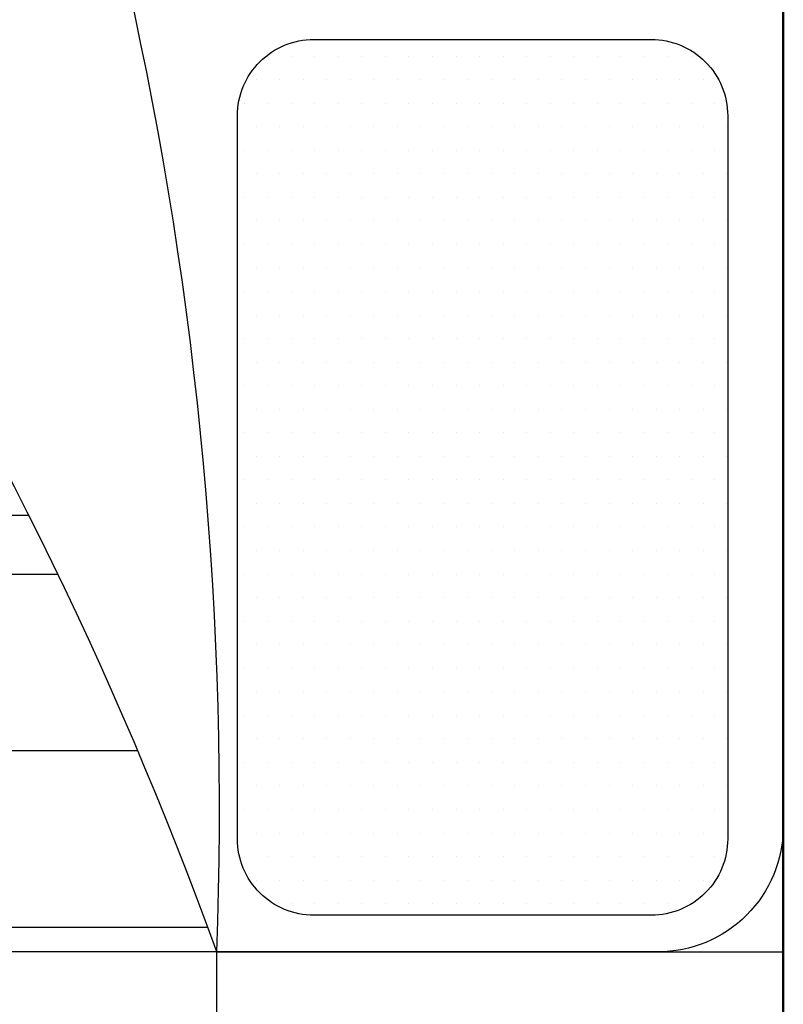
# Model space of a CAD drawing. Units: inches. Extents: x 3064 to 19385, y 846 to 15425.
# Tile 69 of 108: x 6580 to 6604, y 1624 to 1655. Entities that reach past the tile are written whole.
import ezdxf

# ---------------------------------------------------------------- set-up
doc = ezdxf.new("R2010")
doc.units = ezdxf.units.IN
doc.layers.add('A-FLOR-FIXT', color=9, linetype='Continuous', lineweight=18)
doc.layers.add('A-WALL', color=7, linetype='Continuous', lineweight=50)
doc.layers.add('BLOCK', color=6, linetype='Continuous')

# ---------------------------------------------------------------- blocks, each defined once
blk = doc.blocks.new('*X6')
at = {"color": 0}
for p, q in [((280.3125, 439.8862), (280.3125, 452.8965)), ((278.9062, 439.4824), (278.9062, 452.3385)), ((277.5, 439.4824), (277.5, 451.7019)), ((277.0312, 439.4824), (277.0312, 451.4714))]:
    blk.add_line(p, q, dxfattribs=at)
blk = doc.blocks.new('*X7')
at = {"color": 0}
for p, q in [((273.9375, 457.03125), (273.9375, 457.03125)), ((274.3125, 457.03125), (274.3125, 457.03125)), ((274.6875, 457.03125), (274.6875, 457.03125)), ((275.0625, 457.03125), (275.0625, 457.03125)), ((275.4375, 457.03125), (275.4375, 457.03125)), ((275.8125, 457.03125), (275.8125, 457.03125)), ((276.1875, 457.03125), (276.1875, 457.03125)), ((276.5625, 457.03125), (276.5625, 457.03125)), ((276.9375, 457.03125), (276.9375, 457.03125)), ((277.3125, 457.03125), (277.3125, 457.03125)), ((277.6875, 457.03125), (277.6875, 457.03125)), ((278.0625, 457.03125), (278.0625, 457.03125)), ((278.4375, 457.03125), (278.4375, 457.03125)), ((278.8125, 457.03125), (278.8125, 457.03125)), ((279.1875, 457.03125), (279.1875, 457.03125)), ((279.5625, 457.03125), (279.5625, 457.03125)), ((273.75, 456.9375), (273.75, 456.9375)), ((274.125, 456.9375), (274.125, 456.9375)), ((274.5, 456.9375), (274.5, 456.9375)), ((274.875, 456.9375), (274.875, 456.9375)), ((275.25, 456.9375), (275.25, 456.9375)), ((275.625, 456.9375), (275.625, 456.9375)), ((276, 456.9375), (276, 456.9375)), ((276.375, 456.9375), (276.375, 456.9375)), ((276.75, 456.9375), (276.75, 456.9375)), ((277.125, 456.9375), (277.125, 456.9375)), ((277.5, 456.9375), (277.5, 456.9375)), ((277.875, 456.9375), (277.875, 456.9375)), ((278.25, 456.9375), (278.25, 456.9375)), ((278.625, 456.9375), (278.625, 456.9375)), ((279, 456.9375), (279, 456.9375)), ((279.375, 456.9375), (279.375, 456.9375)), ((279.75, 456.9375), (279.75, 456.9375)), ((273.5625, 456.84375), (273.5625, 456.84375)), ((273.9375, 456.84375), (273.9375, 456.84375)), ((274.3125, 456.84375), (274.3125, 456.84375)), ((274.6875, 456.84375), (274.6875, 456.84375)), ((275.0625, 456.84375), (275.0625, 456.84375)), ((275.4375, 456.84375), (275.4375, 456.84375)), ((275.8125, 456.84375), (275.8125, 456.84375)), ((276.1875, 456.84375), (276.1875, 456.84375)), ((276.5625, 456.84375), (276.5625, 456.84375)), ((276.9375, 456.84375), (276.9375, 456.84375)), ((277.3125, 456.84375), (277.3125, 456.84375)), ((277.6875, 456.84375), (277.6875, 456.84375)), ((278.0625, 456.84375), (278.0625, 456.84375)), ((278.4375, 456.84375), (278.4375, 456.84375)), ((278.8125, 456.84375), (278.8125, 456.84375)), ((279.1875, 456.84375), (279.1875, 456.84375)), ((279.5625, 456.84375), (279.5625, 456.84375)), ((279.9375, 456.84375), (279.9375, 456.84375)), ((273.375, 456.75), (273.375, 456.75)), ((273.75, 456.75), (273.75, 456.75)), ((274.125, 456.75), (274.125, 456.75)), ((274.5, 456.75), (274.5, 456.75)), ((274.875, 456.75), (274.875, 456.75)), ((275.25, 456.75), (275.25, 456.75)), ((275.625, 456.75), (275.625, 456.75)), ((276, 456.75), (276, 456.75)), ((276.375, 456.75), (276.375, 456.75)), ((276.75, 456.75), (276.75, 456.75)), ((277.125, 456.75), (277.125, 456.75)), ((277.5, 456.75), (277.5, 456.75)), ((277.875, 456.75), (277.875, 456.75)), ((278.25, 456.75), (278.25, 456.75)), ((278.625, 456.75), (278.625, 456.75)), ((279, 456.75), (279, 456.75)), ((279.375, 456.75), (279.375, 456.75)), ((279.75, 456.75), (279.75, 456.75)), ((280.125, 456.75), (280.125, 456.75)), ((273.5625, 456.65625), (273.5625, 456.65625)), ((273.9375, 456.65625), (273.9375, 456.65625)), ((274.3125, 456.65625), (274.3125, 456.65625)), ((274.6875, 456.65625), (274.6875, 456.65625)), ((275.0625, 456.65625), (275.0625, 456.65625)), ((275.4375, 456.65625), (275.4375, 456.65625)), ((275.8125, 456.65625), (275.8125, 456.65625)), ((276.1875, 456.65625), (276.1875, 456.65625)), ((276.5625, 456.65625), (276.5625, 456.65625)), ((276.9375, 456.65625), (276.9375, 456.65625)), ((277.3125, 456.65625), (277.3125, 456.65625)), ((277.6875, 456.65625), (277.6875, 456.65625)), ((278.0625, 456.65625), (278.0625, 456.65625)), ((278.4375, 456.65625), (278.4375, 456.65625)), ((278.8125, 456.65625), (278.8125, 456.65625)), ((279.1875, 456.65625), (279.1875, 456.65625)), ((279.5625, 456.65625), (279.5625, 456.65625)), ((279.9375, 456.65625), (279.9375, 456.65625)), ((273.375, 456.5625), (273.375, 456.5625)), ((273.75, 456.5625), (273.75, 456.5625)), ((274.125, 456.5625), (274.125, 456.5625)), ((274.5, 456.5625), (274.5, 456.5625)), ((274.875, 456.5625), (274.875, 456.5625)), ((275.25, 456.5625), (275.25, 456.5625)), ((275.625, 456.5625), (275.625, 456.5625)), ((276, 456.5625), (276, 456.5625)), ((276.375, 456.5625), (276.375, 456.5625)), ((276.75, 456.5625), (276.75, 456.5625)), ((277.125, 456.5625), (277.125, 456.5625)), ((277.5, 456.5625), (277.5, 456.5625)), ((277.875, 456.5625), (277.875, 456.5625)), ((278.25, 456.5625), (278.25, 456.5625)), ((278.625, 456.5625), (278.625, 456.5625)), ((279, 456.5625), (279, 456.5625)), ((279.375, 456.5625), (279.375, 456.5625)), ((279.75, 456.5625), (279.75, 456.5625)), ((280.125, 456.5625), (280.125, 456.5625)), ((273.5625, 456.46875), (273.5625, 456.46875)), ((273.9375, 456.46875), (273.9375, 456.46875)), ((274.3125, 456.46875), (274.3125, 456.46875)), ((274.6875, 456.46875), (274.6875, 456.46875)), ((275.0625, 456.46875), (275.0625, 456.46875)), ((275.4375, 456.46875), (275.4375, 456.46875)), ((275.8125, 456.46875), (275.8125, 456.46875)), ((276.1875, 456.46875), (276.1875, 456.46875)), ((276.5625, 456.46875), (276.5625, 456.46875)), ((276.9375, 456.46875), (276.9375, 456.46875)), ((277.3125, 456.46875), (277.3125, 456.46875)), ((277.6875, 456.46875), (277.6875, 456.46875)), ((278.0625, 456.46875), (278.0625, 456.46875)), ((278.4375, 456.46875), (278.4375, 456.46875)), ((278.8125, 456.46875), (278.8125, 456.46875)), ((279.1875, 456.46875), (279.1875, 456.46875)), ((279.5625, 456.46875), (279.5625, 456.46875)), ((279.9375, 456.46875), (279.9375, 456.46875)), ((273.375, 456.375), (273.375, 456.375)), ((273.75, 456.375), (273.75, 456.375)), ((274.125, 456.375), (274.125, 456.375)), ((274.5, 456.375), (274.5, 456.375)), ((274.875, 456.375), (274.875, 456.375)), ((275.25, 456.375), (275.25, 456.375)), ((275.625, 456.375), (275.625, 456.375)), ((276, 456.375), (276, 456.375)), ((276.375, 456.375), (276.375, 456.375)), ((276.75, 456.375), (276.75, 456.375)), ((277.125, 456.375), (277.125, 456.375)), ((277.5, 456.375), (277.5, 456.375)), ((277.875, 456.375), (277.875, 456.375)), ((278.25, 456.375), (278.25, 456.375)), ((278.625, 456.375), (278.625, 456.375)), ((279, 456.375), (279, 456.375)), ((279.375, 456.375), (279.375, 456.375)), ((279.75, 456.375), (279.75, 456.375)), ((280.125, 456.375), (280.125, 456.375)), ((273.5625, 456.28125), (273.5625, 456.28125)), ((273.9375, 456.28125), (273.9375, 456.28125)), ((274.3125, 456.28125), (274.3125, 456.28125)), ((274.6875, 456.28125), (274.6875, 456.28125)), ((275.0625, 456.28125), (275.0625, 456.28125)), ((275.4375, 456.28125), (275.4375, 456.28125)), ((275.8125, 456.28125), (275.8125, 456.28125)), ((276.1875, 456.28125), (276.1875, 456.28125)), ((276.5625, 456.28125), (276.5625, 456.28125)), ((276.9375, 456.28125), (276.9375, 456.28125)), ((277.3125, 456.28125), (277.3125, 456.28125)), ((277.6875, 456.28125), (277.6875, 456.28125)), ((278.0625, 456.28125), (278.0625, 456.28125)), ((278.4375, 456.28125), (278.4375, 456.28125)), ((278.8125, 456.28125), (278.8125, 456.28125)), ((279.1875, 456.28125), (279.1875, 456.28125)), ((279.5625, 456.28125), (279.5625, 456.28125)), ((279.9375, 456.28125), (279.9375, 456.28125)), ((273.375, 456.1875), (273.375, 456.1875)), ((273.75, 456.1875), (273.75, 456.1875)), ((274.125, 456.1875), (274.125, 456.1875)), ((274.5, 456.1875), (274.5, 456.1875)), ((274.875, 456.1875), (274.875, 456.1875)), ((275.25, 456.1875), (275.25, 456.1875)), ((275.625, 456.1875), (275.625, 456.1875)), ((276, 456.1875), (276, 456.1875)), ((276.375, 456.1875), (276.375, 456.1875)), ((276.75, 456.1875), (276.75, 456.1875)), ((277.125, 456.1875), (277.125, 456.1875)), ((277.5, 456.1875), (277.5, 456.1875)), ((277.875, 456.1875), (277.875, 456.1875)), ((278.25, 456.1875), (278.25, 456.1875)), ((278.625, 456.1875), (278.625, 456.1875)), ((279, 456.1875), (279, 456.1875)), ((279.375, 456.1875), (279.375, 456.1875)), ((279.75, 456.1875), (279.75, 456.1875)), ((280.125, 456.1875), (280.125, 456.1875)), ((273.5625, 456.09375), (273.5625, 456.09375)), ((273.9375, 456.09375), (273.9375, 456.09375)), ((274.3125, 456.09375), (274.3125, 456.09375)), ((274.6875, 456.09375), (274.6875, 456.09375)), ((275.0625, 456.09375), (275.0625, 456.09375)), ((275.4375, 456.09375), (275.4375, 456.09375)), ((275.8125, 456.09375), (275.8125, 456.09375)), ((276.1875, 456.09375), (276.1875, 456.09375)), ((276.5625, 456.09375), (276.5625, 456.09375)), ((276.9375, 456.09375), (276.9375, 456.09375)), ((277.3125, 456.09375), (277.3125, 456.09375)), ((277.6875, 456.09375), (277.6875, 456.09375)), ((278.0625, 456.09375), (278.0625, 456.09375)), ((278.4375, 456.09375), (278.4375, 456.09375)), ((278.8125, 456.09375), (278.8125, 456.09375)), ((279.1875, 456.09375), (279.1875, 456.09375)), ((279.5625, 456.09375), (279.5625, 456.09375)), ((279.9375, 456.09375), (279.9375, 456.09375)), ((273.375, 456), (273.375, 456)), ((273.75, 456), (273.75, 456)), ((274.125, 456), (274.125, 456)), ((274.5, 456), (274.5, 456)), ((274.875, 456), (274.875, 456)), ((275.25, 456), (275.25, 456)), ((275.625, 456), (275.625, 456)), ((276, 456), (276, 456)), ((276.375, 456), (276.375, 456)), ((276.75, 456), (276.75, 456)), ((277.125, 456), (277.125, 456)), ((277.5, 456), (277.5, 456)), ((277.875, 456), (277.875, 456)), ((278.25, 456), (278.25, 456)), ((278.625, 456), (278.625, 456)), ((279, 456), (279, 456)), ((279.375, 456), (279.375, 456)), ((279.75, 456), (279.75, 456)), ((280.125, 456), (280.125, 456)), ((273.5625, 455.90625), (273.5625, 455.90625)), ((273.9375, 455.90625), (273.9375, 455.90625)), ((274.3125, 455.90625), (274.3125, 455.90625)), ((274.6875, 455.90625), (274.6875, 455.90625)), ((275.0625, 455.90625), (275.0625, 455.90625)), ((275.4375, 455.90625), (275.4375, 455.90625)), ((275.8125, 455.90625), (275.8125, 455.90625)), ((276.1875, 455.90625), (276.1875, 455.90625)), ((276.5625, 455.90625), (276.5625, 455.90625)), ((276.9375, 455.90625), (276.9375, 455.90625)), ((277.3125, 455.90625), (277.3125, 455.90625)), ((277.6875, 455.90625), (277.6875, 455.90625)), ((278.0625, 455.90625), (278.0625, 455.90625)), ((278.4375, 455.90625), (278.4375, 455.90625)), ((278.8125, 455.90625), (278.8125, 455.90625)), ((279.1875, 455.90625), (279.1875, 455.90625)), ((279.5625, 455.90625), (279.5625, 455.90625)), ((279.9375, 455.90625), (279.9375, 455.90625)), ((273.375, 455.8125), (273.375, 455.8125)), ((273.75, 455.8125), (273.75, 455.8125)), ((274.125, 455.8125), (274.125, 455.8125)), ((274.5, 455.8125), (274.5, 455.8125)), ((274.875, 455.8125), (274.875, 455.8125)), ((275.25, 455.8125), (275.25, 455.8125)), ((275.625, 455.8125), (275.625, 455.8125)), ((276, 455.8125), (276, 455.8125)), ((276.375, 455.8125), (276.375, 455.8125)), ((276.75, 455.8125), (276.75, 455.8125)), ((277.125, 455.8125), (277.125, 455.8125)), ((277.5, 455.8125), (277.5, 455.8125)), ((277.875, 455.8125), (277.875, 455.8125)), ((278.25, 455.8125), (278.25, 455.8125)), ((278.625, 455.8125), (278.625, 455.8125)), ((279, 455.8125), (279, 455.8125)), ((279.375, 455.8125), (279.375, 455.8125)), ((279.75, 455.8125), (279.75, 455.8125)), ((280.125, 455.8125), (280.125, 455.8125)), ((273.5625, 455.71875), (273.5625, 455.71875)), ((273.9375, 455.71875), (273.9375, 455.71875)), ((274.3125, 455.71875), (274.3125, 455.71875)), ((274.6875, 455.71875), (274.6875, 455.71875)), ((275.0625, 455.71875), (275.0625, 455.71875)), ((275.4375, 455.71875), (275.4375, 455.71875)), ((275.8125, 455.71875), (275.8125, 455.71875)), ((276.1875, 455.71875), (276.1875, 455.71875)), ((276.5625, 455.71875), (276.5625, 455.71875)), ((276.9375, 455.71875), (276.9375, 455.71875)), ((277.3125, 455.71875), (277.3125, 455.71875)), ((277.6875, 455.71875), (277.6875, 455.71875)), ((278.0625, 455.71875), (278.0625, 455.71875)), ((278.4375, 455.71875), (278.4375, 455.71875)), ((278.8125, 455.71875), (278.8125, 455.71875)), ((279.1875, 455.71875), (279.1875, 455.71875)), ((279.5625, 455.71875), (279.5625, 455.71875)), ((279.9375, 455.71875), (279.9375, 455.71875)), ((273.375, 455.625), (273.375, 455.625)), ((273.75, 455.625), (273.75, 455.625)), ((274.125, 455.625), (274.125, 455.625)), ((274.5, 455.625), (274.5, 455.625)), ((274.875, 455.625), (274.875, 455.625)), ((275.25, 455.625), (275.25, 455.625)), ((275.625, 455.625), (275.625, 455.625)), ((276, 455.625), (276, 455.625)), ((276.375, 455.625), (276.375, 455.625)), ((276.75, 455.625), (276.75, 455.625)), ((277.125, 455.625), (277.125, 455.625)), ((277.5, 455.625), (277.5, 455.625)), ((277.875, 455.625), (277.875, 455.625)), ((278.25, 455.625), (278.25, 455.625)), ((278.625, 455.625), (278.625, 455.625)), ((279, 455.625), (279, 455.625)), ((279.375, 455.625), (279.375, 455.625)), ((279.75, 455.625), (279.75, 455.625)), ((280.125, 455.625), (280.125, 455.625)), ((273.5625, 455.53125), (273.5625, 455.53125)), ((273.9375, 455.53125), (273.9375, 455.53125)), ((274.3125, 455.53125), (274.3125, 455.53125)), ((274.6875, 455.53125), (274.6875, 455.53125)), ((275.0625, 455.53125), (275.0625, 455.53125)), ((275.4375, 455.53125), (275.4375, 455.53125)), ((275.8125, 455.53125), (275.8125, 455.53125)), ((276.1875, 455.53125), (276.1875, 455.53125)), ((276.5625, 455.53125), (276.5625, 455.53125)), ((276.9375, 455.53125), (276.9375, 455.53125)), ((277.3125, 455.53125), (277.3125, 455.53125)), ((277.6875, 455.53125), (277.6875, 455.53125)), ((278.0625, 455.53125), (278.0625, 455.53125)), ((278.4375, 455.53125), (278.4375, 455.53125)), ((278.8125, 455.53125), (278.8125, 455.53125)), ((279.1875, 455.53125), (279.1875, 455.53125)), ((279.5625, 455.53125), (279.5625, 455.53125)), ((279.9375, 455.53125), (279.9375, 455.53125)), ((273.375, 455.4375), (273.375, 455.4375)), ((273.75, 455.4375), (273.75, 455.4375)), ((274.125, 455.4375), (274.125, 455.4375)), ((274.5, 455.4375), (274.5, 455.4375)), ((274.875, 455.4375), (274.875, 455.4375)), ((275.25, 455.4375), (275.25, 455.4375)), ((275.625, 455.4375), (275.625, 455.4375)), ((276, 455.4375), (276, 455.4375)), ((276.375, 455.4375), (276.375, 455.4375)), ((276.75, 455.4375), (276.75, 455.4375)), ((277.125, 455.4375), (277.125, 455.4375)), ((277.5, 455.4375), (277.5, 455.4375)), ((277.875, 455.4375), (277.875, 455.4375)), ((278.25, 455.4375), (278.25, 455.4375)), ((278.625, 455.4375), (278.625, 455.4375)), ((279, 455.4375), (279, 455.4375)), ((279.375, 455.4375), (279.375, 455.4375)), ((279.75, 455.4375), (279.75, 455.4375)), ((280.125, 455.4375), (280.125, 455.4375)), ((273.5625, 455.34375), (273.5625, 455.34375)), ((273.9375, 455.34375), (273.9375, 455.34375)), ((274.3125, 455.34375), (274.3125, 455.34375)), ((274.6875, 455.34375), (274.6875, 455.34375)), ((275.0625, 455.34375), (275.0625, 455.34375)), ((275.4375, 455.34375), (275.4375, 455.34375)), ((275.8125, 455.34375), (275.8125, 455.34375)), ((276.1875, 455.34375), (276.1875, 455.34375)), ((276.5625, 455.34375), (276.5625, 455.34375)), ((276.9375, 455.34375), (276.9375, 455.34375)), ((277.3125, 455.34375), (277.3125, 455.34375)), ((277.6875, 455.34375), (277.6875, 455.34375)), ((278.0625, 455.34375), (278.0625, 455.34375)), ((278.4375, 455.34375), (278.4375, 455.34375)), ((278.8125, 455.34375), (278.8125, 455.34375)), ((279.1875, 455.34375), (279.1875, 455.34375)), ((279.5625, 455.34375), (279.5625, 455.34375)), ((279.9375, 455.34375), (279.9375, 455.34375)), ((273.375, 455.25), (273.375, 455.25)), ((273.75, 455.25), (273.75, 455.25)), ((274.125, 455.25), (274.125, 455.25)), ((274.5, 455.25), (274.5, 455.25)), ((274.875, 455.25), (274.875, 455.25)), ((275.25, 455.25), (275.25, 455.25)), ((275.625, 455.25), (275.625, 455.25)), ((276, 455.25), (276, 455.25)), ((276.375, 455.25), (276.375, 455.25)), ((276.75, 455.25), (276.75, 455.25)), ((277.125, 455.25), (277.125, 455.25)), ((277.5, 455.25), (277.5, 455.25)), ((277.875, 455.25), (277.875, 455.25)), ((278.25, 455.25), (278.25, 455.25)), ((278.625, 455.25), (278.625, 455.25)), ((279, 455.25), (279, 455.25)), ((279.375, 455.25), (279.375, 455.25)), ((279.75, 455.25), (279.75, 455.25)), ((280.125, 455.25), (280.125, 455.25)), ((273.5625, 455.15625), (273.5625, 455.15625)), ((273.9375, 455.15625), (273.9375, 455.15625)), ((274.3125, 455.15625), (274.3125, 455.15625)), ((274.6875, 455.15625), (274.6875, 455.15625)), ((275.0625, 455.15625), (275.0625, 455.15625)), ((275.4375, 455.15625), (275.4375, 455.15625)), ((275.8125, 455.15625), (275.8125, 455.15625)), ((276.1875, 455.15625), (276.1875, 455.15625)), ((276.5625, 455.15625), (276.5625, 455.15625)), ((276.9375, 455.15625), (276.9375, 455.15625)), ((277.3125, 455.15625), (277.3125, 455.15625)), ((277.6875, 455.15625), (277.6875, 455.15625)), ((278.0625, 455.15625), (278.0625, 455.15625)), ((278.4375, 455.15625), (278.4375, 455.15625)), ((278.8125, 455.15625), (278.8125, 455.15625)), ((279.1875, 455.15625), (279.1875, 455.15625)), ((279.5625, 455.15625), (279.5625, 455.15625)), ((279.9375, 455.15625), (279.9375, 455.15625)), ((273.375, 455.0625), (273.375, 455.0625)), ((273.75, 455.0625), (273.75, 455.0625)), ((274.125, 455.0625), (274.125, 455.0625)), ((274.5, 455.0625), (274.5, 455.0625)), ((274.875, 455.0625), (274.875, 455.0625)), ((275.25, 455.0625), (275.25, 455.0625)), ((275.625, 455.0625), (275.625, 455.0625)), ((276, 455.0625), (276, 455.0625)), ((276.375, 455.0625), (276.375, 455.0625)), ((276.75, 455.0625), (276.75, 455.0625)), ((277.125, 455.0625), (277.125, 455.0625)), ((277.5, 455.0625), (277.5, 455.0625)), ((277.875, 455.0625), (277.875, 455.0625)), ((278.25, 455.0625), (278.25, 455.0625)), ((278.625, 455.0625), (278.625, 455.0625)), ((279, 455.0625), (279, 455.0625)), ((279.375, 455.0625), (279.375, 455.0625)), ((279.75, 455.0625), (279.75, 455.0625)), ((280.125, 455.0625), (280.125, 455.0625)), ((273.5625, 454.96875), (273.5625, 454.96875)), ((273.9375, 454.96875), (273.9375, 454.96875)), ((274.3125, 454.96875), (274.3125, 454.96875)), ((274.6875, 454.96875), (274.6875, 454.96875)), ((275.0625, 454.96875), (275.0625, 454.96875)), ((275.4375, 454.96875), (275.4375, 454.96875)), ((275.8125, 454.96875), (275.8125, 454.96875)), ((276.1875, 454.96875), (276.1875, 454.96875)), ((276.5625, 454.96875), (276.5625, 454.96875)), ((276.9375, 454.96875), (276.9375, 454.96875)), ((277.3125, 454.96875), (277.3125, 454.96875)), ((277.6875, 454.96875), (277.6875, 454.96875)), ((278.0625, 454.96875), (278.0625, 454.96875)), ((278.4375, 454.96875), (278.4375, 454.96875)), ((278.8125, 454.96875), (278.8125, 454.96875)), ((279.1875, 454.96875), (279.1875, 454.96875)), ((279.5625, 454.96875), (279.5625, 454.96875)), ((279.9375, 454.96875), (279.9375, 454.96875)), ((273.375, 454.875), (273.375, 454.875)), ((273.75, 454.875), (273.75, 454.875)), ((274.125, 454.875), (274.125, 454.875)), ((274.5, 454.875), (274.5, 454.875)), ((274.875, 454.875), (274.875, 454.875)), ((275.25, 454.875), (275.25, 454.875)), ((275.625, 454.875), (275.625, 454.875)), ((276, 454.875), (276, 454.875)), ((276.375, 454.875), (276.375, 454.875)), ((276.75, 454.875), (276.75, 454.875)), ((277.125, 454.875), (277.125, 454.875)), ((277.5, 454.875), (277.5, 454.875)), ((277.875, 454.875), (277.875, 454.875)), ((278.25, 454.875), (278.25, 454.875)), ((278.625, 454.875), (278.625, 454.875)), ((279, 454.875), (279, 454.875)), ((279.375, 454.875), (279.375, 454.875)), ((279.75, 454.875), (279.75, 454.875)), ((280.125, 454.875), (280.125, 454.875)), ((273.5625, 454.78125), (273.5625, 454.78125)), ((273.9375, 454.78125), (273.9375, 454.78125)), ((274.3125, 454.78125), (274.3125, 454.78125)), ((274.6875, 454.78125), (274.6875, 454.78125)), ((275.0625, 454.78125), (275.0625, 454.78125)), ((275.4375, 454.78125), (275.4375, 454.78125)), ((275.8125, 454.78125), (275.8125, 454.78125)), ((276.1875, 454.78125), (276.1875, 454.78125)), ((276.5625, 454.78125), (276.5625, 454.78125)), ((276.9375, 454.78125), (276.9375, 454.78125)), ((277.3125, 454.78125), (277.3125, 454.78125)), ((277.6875, 454.78125), (277.6875, 454.78125)), ((278.0625, 454.78125), (278.0625, 454.78125)), ((278.4375, 454.78125), (278.4375, 454.78125)), ((278.8125, 454.78125), (278.8125, 454.78125)), ((279.1875, 454.78125), (279.1875, 454.78125)), ((279.5625, 454.78125), (279.5625, 454.78125)), ((279.9375, 454.78125), (279.9375, 454.78125)), ((273.375, 454.6875), (273.375, 454.6875)), ((273.75, 454.6875), (273.75, 454.6875)), ((274.125, 454.6875), (274.125, 454.6875)), ((274.5, 454.6875), (274.5, 454.6875)), ((274.875, 454.6875), (274.875, 454.6875)), ((275.25, 454.6875), (275.25, 454.6875)), ((275.625, 454.6875), (275.625, 454.6875)), ((276, 454.6875), (276, 454.6875)), ((276.375, 454.6875), (276.375, 454.6875)), ((276.75, 454.6875), (276.75, 454.6875)), ((277.125, 454.6875), (277.125, 454.6875)), ((277.5, 454.6875), (277.5, 454.6875)), ((277.875, 454.6875), (277.875, 454.6875)), ((278.25, 454.6875), (278.25, 454.6875)), ((278.625, 454.6875), (278.625, 454.6875)), ((279, 454.6875), (279, 454.6875)), ((279.375, 454.6875), (279.375, 454.6875)), ((279.75, 454.6875), (279.75, 454.6875)), ((280.125, 454.6875), (280.125, 454.6875)), ((273.5625, 454.59375), (273.5625, 454.59375)), ((273.9375, 454.59375), (273.9375, 454.59375)), ((274.3125, 454.59375), (274.3125, 454.59375)), ((274.6875, 454.59375), (274.6875, 454.59375)), ((275.0625, 454.59375), (275.0625, 454.59375)), ((275.4375, 454.59375), (275.4375, 454.59375)), ((275.8125, 454.59375), (275.8125, 454.59375)), ((276.1875, 454.59375), (276.1875, 454.59375)), ((276.5625, 454.59375), (276.5625, 454.59375)), ((276.9375, 454.59375), (276.9375, 454.59375)), ((277.3125, 454.59375), (277.3125, 454.59375)), ((277.6875, 454.59375), (277.6875, 454.59375)), ((278.0625, 454.59375), (278.0625, 454.59375)), ((278.4375, 454.59375), (278.4375, 454.59375)), ((278.8125, 454.59375), (278.8125, 454.59375)), ((279.1875, 454.59375), (279.1875, 454.59375)), ((279.5625, 454.59375), (279.5625, 454.59375)), ((279.9375, 454.59375), (279.9375, 454.59375)), ((273.375, 454.5), (273.375, 454.5)), ((273.75, 454.5), (273.75, 454.5)), ((274.125, 454.5), (274.125, 454.5)), ((274.5, 454.5), (274.5, 454.5)), ((274.875, 454.5), (274.875, 454.5)), ((275.25, 454.5), (275.25, 454.5)), ((275.625, 454.5), (275.625, 454.5)), ((276, 454.5), (276, 454.5)), ((276.375, 454.5), (276.375, 454.5)), ((276.75, 454.5), (276.75, 454.5)), ((277.125, 454.5), (277.125, 454.5)), ((277.5, 454.5), (277.5, 454.5)), ((277.875, 454.5), (277.875, 454.5)), ((278.25, 454.5), (278.25, 454.5)), ((278.625, 454.5), (278.625, 454.5)), ((279, 454.5), (279, 454.5)), ((279.375, 454.5), (279.375, 454.5)), ((279.75, 454.5), (279.75, 454.5)), ((280.125, 454.5), (280.125, 454.5)), ((273.5625, 454.40625), (273.5625, 454.40625)), ((273.9375, 454.40625), (273.9375, 454.40625)), ((274.3125, 454.40625), (274.3125, 454.40625)), ((274.6875, 454.40625), (274.6875, 454.40625)), ((275.0625, 454.40625), (275.0625, 454.40625)), ((275.4375, 454.40625), (275.4375, 454.40625)), ((275.8125, 454.40625), (275.8125, 454.40625)), ((276.1875, 454.40625), (276.1875, 454.40625)), ((276.5625, 454.40625), (276.5625, 454.40625)), ((276.9375, 454.40625), (276.9375, 454.40625)), ((277.3125, 454.40625), (277.3125, 454.40625)), ((277.6875, 454.40625), (277.6875, 454.40625)), ((278.0625, 454.40625), (278.0625, 454.40625)), ((278.4375, 454.40625), (278.4375, 454.40625)), ((278.8125, 454.40625), (278.8125, 454.40625)), ((279.1875, 454.40625), (279.1875, 454.40625)), ((279.5625, 454.40625), (279.5625, 454.40625)), ((279.9375, 454.40625), (279.9375, 454.40625)), ((273.375, 454.3125), (273.375, 454.3125)), ((273.75, 454.3125), (273.75, 454.3125)), ((274.125, 454.3125), (274.125, 454.3125)), ((274.5, 454.3125), (274.5, 454.3125)), ((274.875, 454.3125), (274.875, 454.3125)), ((275.25, 454.3125), (275.25, 454.3125)), ((275.625, 454.3125), (275.625, 454.3125)), ((276, 454.3125), (276, 454.3125)), ((276.375, 454.3125), (276.375, 454.3125)), ((276.75, 454.3125), (276.75, 454.3125)), ((277.125, 454.3125), (277.125, 454.3125)), ((277.5, 454.3125), (277.5, 454.3125)), ((277.875, 454.3125), (277.875, 454.3125)), ((278.25, 454.3125), (278.25, 454.3125)), ((278.625, 454.3125), (278.625, 454.3125)), ((279, 454.3125), (279, 454.3125)), ((279.375, 454.3125), (279.375, 454.3125)), ((279.75, 454.3125), (279.75, 454.3125)), ((280.125, 454.3125), (280.125, 454.3125)), ((273.5625, 454.21875), (273.5625, 454.21875)), ((273.9375, 454.21875), (273.9375, 454.21875)), ((274.3125, 454.21875), (274.3125, 454.21875)), ((274.6875, 454.21875), (274.6875, 454.21875)), ((275.0625, 454.21875), (275.0625, 454.21875)), ((275.4375, 454.21875), (275.4375, 454.21875)), ((275.8125, 454.21875), (275.8125, 454.21875)), ((276.1875, 454.21875), (276.1875, 454.21875)), ((276.5625, 454.21875), (276.5625, 454.21875)), ((276.9375, 454.21875), (276.9375, 454.21875)), ((277.3125, 454.21875), (277.3125, 454.21875)), ((277.6875, 454.21875), (277.6875, 454.21875)), ((278.0625, 454.21875), (278.0625, 454.21875)), ((278.4375, 454.21875), (278.4375, 454.21875)), ((278.8125, 454.21875), (278.8125, 454.21875)), ((279.1875, 454.21875), (279.1875, 454.21875)), ((279.5625, 454.21875), (279.5625, 454.21875)), ((279.9375, 454.21875), (279.9375, 454.21875)), ((273.375, 454.125), (273.375, 454.125)), ((273.75, 454.125), (273.75, 454.125)), ((274.125, 454.125), (274.125, 454.125)), ((274.5, 454.125), (274.5, 454.125)), ((274.875, 454.125), (274.875, 454.125)), ((275.25, 454.125), (275.25, 454.125)), ((275.625, 454.125), (275.625, 454.125)), ((276, 454.125), (276, 454.125)), ((276.375, 454.125), (276.375, 454.125)), ((276.75, 454.125), (276.75, 454.125)), ((277.125, 454.125), (277.125, 454.125)), ((277.5, 454.125), (277.5, 454.125)), ((277.875, 454.125), (277.875, 454.125)), ((278.25, 454.125), (278.25, 454.125)), ((278.625, 454.125), (278.625, 454.125)), ((279, 454.125), (279, 454.125)), ((279.375, 454.125), (279.375, 454.125)), ((279.75, 454.125), (279.75, 454.125)), ((280.125, 454.125), (280.125, 454.125)), ((273.5625, 454.03125), (273.5625, 454.03125)), ((273.9375, 454.03125), (273.9375, 454.03125)), ((274.3125, 454.03125), (274.3125, 454.03125)), ((274.6875, 454.03125), (274.6875, 454.03125)), ((275.0625, 454.03125), (275.0625, 454.03125)), ((275.4375, 454.03125), (275.4375, 454.03125)), ((275.8125, 454.03125), (275.8125, 454.03125)), ((276.1875, 454.03125), (276.1875, 454.03125)), ((276.5625, 454.03125), (276.5625, 454.03125)), ((276.9375, 454.03125), (276.9375, 454.03125)), ((277.3125, 454.03125), (277.3125, 454.03125)), ((277.6875, 454.03125), (277.6875, 454.03125)), ((278.0625, 454.03125), (278.0625, 454.03125)), ((278.4375, 454.03125), (278.4375, 454.03125)), ((278.8125, 454.03125), (278.8125, 454.03125)), ((279.1875, 454.03125), (279.1875, 454.03125)), ((279.5625, 454.03125), (279.5625, 454.03125)), ((279.9375, 454.03125), (279.9375, 454.03125)), ((273.375, 453.9375), (273.375, 453.9375)), ((273.75, 453.9375), (273.75, 453.9375)), ((274.125, 453.9375), (274.125, 453.9375)), ((274.5, 453.9375), (274.5, 453.9375)), ((274.875, 453.9375), (274.875, 453.9375)), ((275.25, 453.9375), (275.25, 453.9375)), ((275.625, 453.9375), (275.625, 453.9375)), ((276, 453.9375), (276, 453.9375)), ((276.375, 453.9375), (276.375, 453.9375)), ((276.75, 453.9375), (276.75, 453.9375)), ((277.125, 453.9375), (277.125, 453.9375)), ((277.5, 453.9375), (277.5, 453.9375)), ((277.875, 453.9375), (277.875, 453.9375)), ((278.25, 453.9375), (278.25, 453.9375)), ((278.625, 453.9375), (278.625, 453.9375)), ((279, 453.9375), (279, 453.9375)), ((279.375, 453.9375), (279.375, 453.9375)), ((279.75, 453.9375), (279.75, 453.9375)), ((280.125, 453.9375), (280.125, 453.9375)), ((273.5625, 453.84375), (273.5625, 453.84375)), ((273.9375, 453.84375), (273.9375, 453.84375)), ((274.3125, 453.84375), (274.3125, 453.84375)), ((274.6875, 453.84375), (274.6875, 453.84375)), ((275.0625, 453.84375), (275.0625, 453.84375)), ((275.4375, 453.84375), (275.4375, 453.84375)), ((275.8125, 453.84375), (275.8125, 453.84375)), ((276.1875, 453.84375), (276.1875, 453.84375)), ((276.5625, 453.84375), (276.5625, 453.84375)), ((276.9375, 453.84375), (276.9375, 453.84375)), ((277.3125, 453.84375), (277.3125, 453.84375)), ((277.6875, 453.84375), (277.6875, 453.84375)), ((278.0625, 453.84375), (278.0625, 453.84375)), ((278.4375, 453.84375), (278.4375, 453.84375)), ((278.8125, 453.84375), (278.8125, 453.84375)), ((279.1875, 453.84375), (279.1875, 453.84375)), ((279.5625, 453.84375), (279.5625, 453.84375)), ((279.9375, 453.84375), (279.9375, 453.84375)), ((273.375, 453.75), (273.375, 453.75)), ((273.75, 453.75), (273.75, 453.75)), ((274.125, 453.75), (274.125, 453.75)), ((274.5, 453.75), (274.5, 453.75)), ((274.875, 453.75), (274.875, 453.75)), ((275.25, 453.75), (275.25, 453.75)), ((275.625, 453.75), (275.625, 453.75)), ((276, 453.75), (276, 453.75)), ((276.375, 453.75), (276.375, 453.75)), ((276.75, 453.75), (276.75, 453.75)), ((277.125, 453.75), (277.125, 453.75)), ((277.5, 453.75), (277.5, 453.75)), ((277.875, 453.75), (277.875, 453.75)), ((278.25, 453.75), (278.25, 453.75)), ((278.625, 453.75), (278.625, 453.75)), ((279, 453.75), (279, 453.75)), ((279.375, 453.75), (279.375, 453.75)), ((279.75, 453.75), (279.75, 453.75)), ((280.125, 453.75), (280.125, 453.75)), ((273.5625, 453.65625), (273.5625, 453.65625)), ((273.9375, 453.65625), (273.9375, 453.65625)), ((274.3125, 453.65625), (274.3125, 453.65625)), ((274.6875, 453.65625), (274.6875, 453.65625)), ((275.0625, 453.65625), (275.0625, 453.65625)), ((275.4375, 453.65625), (275.4375, 453.65625)), ((275.8125, 453.65625), (275.8125, 453.65625)), ((276.1875, 453.65625), (276.1875, 453.65625)), ((276.5625, 453.65625), (276.5625, 453.65625)), ((276.9375, 453.65625), (276.9375, 453.65625)), ((277.3125, 453.65625), (277.3125, 453.65625)), ((277.6875, 453.65625), (277.6875, 453.65625)), ((278.0625, 453.65625), (278.0625, 453.65625)), ((278.4375, 453.65625), (278.4375, 453.65625)), ((278.8125, 453.65625), (278.8125, 453.65625)), ((279.1875, 453.65625), (279.1875, 453.65625)), ((279.5625, 453.65625), (279.5625, 453.65625)), ((279.9375, 453.65625), (279.9375, 453.65625)), ((273.375, 453.5625), (273.375, 453.5625)), ((273.75, 453.5625), (273.75, 453.5625)), ((274.125, 453.5625), (274.125, 453.5625)), ((274.5, 453.5625), (274.5, 453.5625)), ((274.875, 453.5625), (274.875, 453.5625)), ((275.25, 453.5625), (275.25, 453.5625)), ((275.625, 453.5625), (275.625, 453.5625)), ((276, 453.5625), (276, 453.5625)), ((276.375, 453.5625), (276.375, 453.5625)), ((276.75, 453.5625), (276.75, 453.5625)), ((277.125, 453.5625), (277.125, 453.5625)), ((277.5, 453.5625), (277.5, 453.5625)), ((277.875, 453.5625), (277.875, 453.5625)), ((278.25, 453.5625), (278.25, 453.5625)), ((278.625, 453.5625), (278.625, 453.5625)), ((279, 453.5625), (279, 453.5625)), ((279.375, 453.5625), (279.375, 453.5625)), ((279.75, 453.5625), (279.75, 453.5625)), ((280.125, 453.5625), (280.125, 453.5625)), ((273.5625, 453.46875), (273.5625, 453.46875)), ((273.9375, 453.46875), (273.9375, 453.46875)), ((274.3125, 453.46875), (274.3125, 453.46875)), ((274.6875, 453.46875), (274.6875, 453.46875)), ((275.0625, 453.46875), (275.0625, 453.46875)), ((275.4375, 453.46875), (275.4375, 453.46875)), ((275.8125, 453.46875), (275.8125, 453.46875)), ((276.1875, 453.46875), (276.1875, 453.46875)), ((276.5625, 453.46875), (276.5625, 453.46875)), ((276.9375, 453.46875), (276.9375, 453.46875)), ((277.3125, 453.46875), (277.3125, 453.46875)), ((277.6875, 453.46875), (277.6875, 453.46875)), ((278.0625, 453.46875), (278.0625, 453.46875)), ((278.4375, 453.46875), (278.4375, 453.46875)), ((278.8125, 453.46875), (278.8125, 453.46875)), ((279.1875, 453.46875), (279.1875, 453.46875)), ((279.5625, 453.46875), (279.5625, 453.46875)), ((279.9375, 453.46875), (279.9375, 453.46875)), ((273.375, 453.375), (273.375, 453.375)), ((273.75, 453.375), (273.75, 453.375)), ((274.125, 453.375), (274.125, 453.375)), ((274.5, 453.375), (274.5, 453.375)), ((274.875, 453.375), (274.875, 453.375)), ((275.25, 453.375), (275.25, 453.375)), ((275.625, 453.375), (275.625, 453.375)), ((276, 453.375), (276, 453.375)), ((276.375, 453.375), (276.375, 453.375)), ((276.75, 453.375), (276.75, 453.375)), ((277.125, 453.375), (277.125, 453.375)), ((277.5, 453.375), (277.5, 453.375)), ((277.875, 453.375), (277.875, 453.375)), ((278.25, 453.375), (278.25, 453.375)), ((278.625, 453.375), (278.625, 453.375)), ((279, 453.375), (279, 453.375)), ((279.375, 453.375), (279.375, 453.375)), ((279.75, 453.375), (279.75, 453.375)), ((273.5625, 453.28125), (273.5625, 453.28125)), ((273.9375, 453.28125), (273.9375, 453.28125)), ((274.3125, 453.28125), (274.3125, 453.28125)), ((274.6875, 453.28125), (274.6875, 453.28125)), ((275.0625, 453.28125), (275.0625, 453.28125)), ((275.4375, 453.28125), (275.4375, 453.28125)), ((275.8125, 453.28125), (275.8125, 453.28125)), ((276.1875, 453.28125), (276.1875, 453.28125)), ((276.5625, 453.28125), (276.5625, 453.28125)), ((276.9375, 453.28125), (276.9375, 453.28125)), ((277.3125, 453.28125), (277.3125, 453.28125)), ((277.6875, 453.28125), (277.6875, 453.28125)), ((278.0625, 453.28125), (278.0625, 453.28125)), ((278.4375, 453.28125), (278.4375, 453.28125)), ((278.8125, 453.28125), (278.8125, 453.28125)), ((279.1875, 453.28125), (279.1875, 453.28125)), ((279.5625, 453.28125), (279.5625, 453.28125)), ((279.9375, 453.28125), (279.9375, 453.28125)), ((273.75, 453.1875), (273.75, 453.1875)), ((274.125, 453.1875), (274.125, 453.1875)), ((274.5, 453.1875), (274.5, 453.1875)), ((274.875, 453.1875), (274.875, 453.1875)), ((275.25, 453.1875), (275.25, 453.1875)), ((275.625, 453.1875), (275.625, 453.1875)), ((276, 453.1875), (276, 453.1875)), ((276.375, 453.1875), (276.375, 453.1875)), ((276.75, 453.1875), (276.75, 453.1875)), ((277.125, 453.1875), (277.125, 453.1875)), ((277.5, 453.1875), (277.5, 453.1875)), ((277.875, 453.1875), (277.875, 453.1875)), ((278.25, 453.1875), (278.25, 453.1875)), ((278.625, 453.1875), (278.625, 453.1875)), ((279, 453.1875), (279, 453.1875)), ((279.375, 453.1875), (279.375, 453.1875)), ((279.75, 453.1875), (279.75, 453.1875))]:
    blk.add_line(p, q, dxfattribs=at)
blk = doc.blocks.new('A$C52E67D0D')
at = {"layer": 'BLOCK'}
for points in [[(1901, 0), (601, 0, -0.414214), (501, 100), (501, 1700, -0.414214), (601, 1800), (1901, 1800, -0.414214), (2001, 1700), (2001, 100, -0.414214)], [(1910.98, 1365.08), (1335.04, 1365.08, -0.414214), (1274.19, 1425.93), (1274.19, 1694.83, -0.414214), (1335.04, 1755.67), (1910.98, 1755.67, -0.414214), (1971.82, 1694.83), (1971.82, 1425.93, -0.414214)]]:
    blk.add_lwpolyline(points, format="xyb", close=True, dxfattribs=at)
blk.add_lwpolyline([(2001, 1348.63), (2001, 1799.63), (2502, 1799.63), (2502, 1348.63)], close=True, dxfattribs=at)
for centre, radius, start, end in [((1888.63, -1664.54), 3015.26, 87.86419, 117.40011), ((3101.01, -1685.8), 3227.66, 109.92605, 135.39771)]:
    blk.add_arc(centre, radius, start, end, dxfattribs=at)
at = {"layer": 'BLOCK', "xscale": 100, "yscale": 100, "zscale": 100}
for name in ['*X7', '*X6']:
    blk.add_blockref(name, (-26049.96, -43948.24), dxfattribs=at)

msp = doc.modelspace()

# ---------------------------------------------------------------- linework, layer by layer
at = {"layer": 'A-WALL'}
msp.add_line((6604.034, 1735.989), (6604.034, 1573.989), dxfattribs=at)

# ---------------------------------------------------------------- block references
at = {"layer": 'A-FLOR-FIXT', "xscale": 0.039370099999992, "yscale": 0.039370099999992, "zscale": 0.039370099999992, "rotation": 270}
msp.add_blockref('A$C52E67D0D', (6533.167, 1704.241), dxfattribs=at)

doc.saveas('drawing.dxf')
